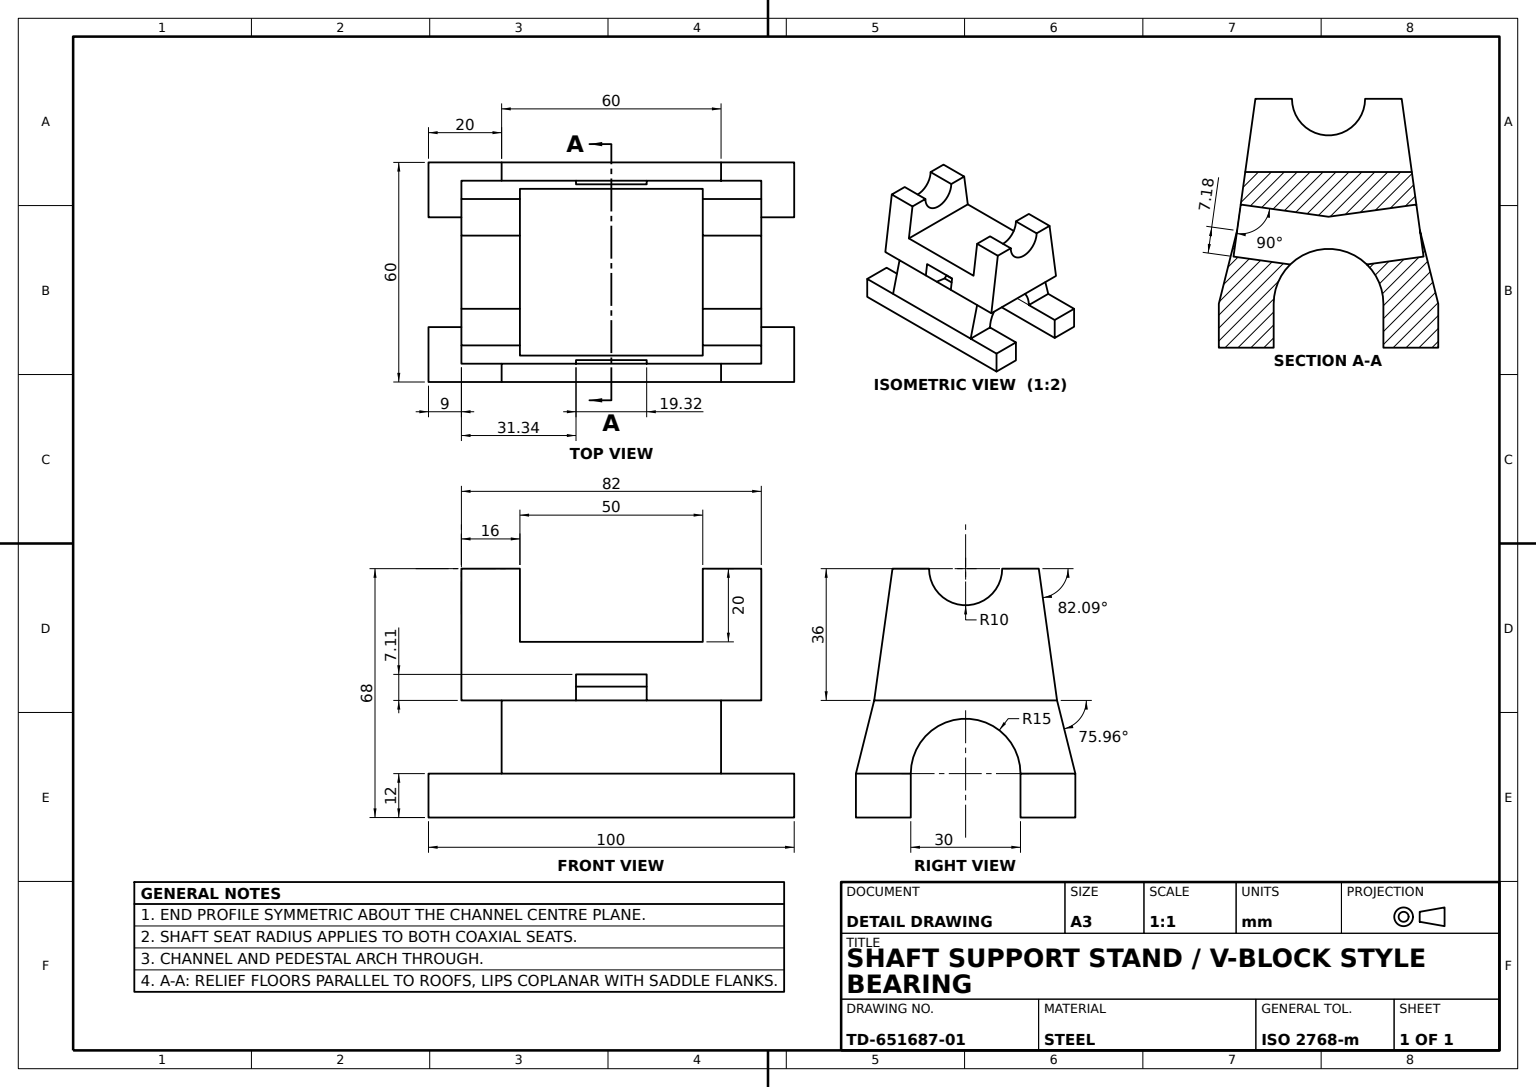
SolidWorks part; units mm, degrees
material "Plain Carbon Steel"
ref_plane "Front Plane" through (0, 0, 0) normal (0, 0, 1) x (1, 0, 0)
ref_plane "Top Plane" through (0, 0, 0) normal (0, 1, 0) x (1, 0, 0)
ref_plane "Right Plane" through (0, 0, 0) normal (1, 0, 0) x (0, 0, -1)
sketch "Base Profile Sketch" plane through (0, 0, 0) normal (0, 1, 0) x (1, 0, 0)
  line L0 (0, 0) -> (30, 0)
  line L1 (30, 0) -> (30, 100)
  line L2 (30, 100) -> (-30, 100)
  line L3 (-30, 100) -> (-30, 0)
  line L4 (-30, 0) -> (0, 0)
  dimension "D1" = 60
  dimension "D2" = 100
  dimension "D3" = 30
extrude "Base Block" add sketch "Base Profile Sketch" along normal blind 12
sketch "Base Channel Sketch" plane through (0, 12, 0) normal (0, 1, 0) x (1, 0, 0)
  line L0 (0, 0) -> (15, 0)
  line L1 (-30, 0) -> (30, 0) construction
  line L2 (15, 0) -> (15, 100)
  line L3 (30, 100) -> (-30, 100) construction
  line L4 (15, 100) -> (-15, 100)
  line L5 (-15, 100) -> (-15, 0)
  line L6 (-15, 0) -> (0, 0)
  dimension "D1" = 30
  dimension "D2" = 15
extrude "Base Channel Cut 30x15" cut sketch "Base Channel Sketch" against normal blind 73
ref_plane "Pedestal Sketch Plane" through (0, 0, -20) normal (0, 0, 1) x (1, 0, 0)
sketch "Pedestal Profile Sketch" plane through (0, 0, -20) normal (0, 0, 1) x (1, 0, 0)
  line L1 (0, 32) -> (25, 32)
  line L2 (25, 32) -> (30, 12)
  line L3 (15, 12) -> (30, 12) construction
  line L4 (0, 32) -> (-25, 32)
  line L5 (-25, 32) -> (-30, 12)
  line L6 (15, 12) -> (30, 12)
  line L7 (-30, 12) -> (-15, 12)
  arc A0 (15, 12) -> (-15, 12) centre (0, 12) ccw
  dimension "D1" = 15
  dimension "D2" = 20
  dimension "D3" = 28.072
  dimension "D4" = 32.0147
  dimension "D5" = 5
  dimension "D6" = 30
  dimension "D7" = 60
extrude "Tapered Pedestal" add sketch "Pedestal Profile Sketch" against normal blind 60
ref_plane "Saddle Sketch Plane" through (0, 0, -9) normal (0, 0, 1) x (1, 0, 0)
sketch "Saddle Profile Sketch" plane through (0, 0, -9) normal (0, 0, 1) x (1, 0, 0)
  line L0 (15, 12) -> (30, 12) construction
  line L1 (25, 32) -> (-25, 32) construction
  line L2 (10, 68) -> (20, 68)
  line L3 (20, 68) -> (25, 32)
  line L4 (25, 32) -> (-10.5729, 32)
  line L5 (-10, 68) -> (-20, 68)
  line L6 (-20, 68) -> (-25, 32)
  line L7 (-25, 32) -> (-10.5729, 32)
  arc A0 (-10, 68) -> (10, 68) centre (0, 68) ccw
  dimension "D1" = 36
  dimension "D3" = 10
  dimension "D2" = 36
  dimension "D4" = 20
  dimension "D5" = 68
  dimension "D6" = 56
  dimension "D7" = 15.814
  dimension "D8" = 10.5729
extrude "Saddle Body" add sketch "Saddle Profile Sketch" against normal blind 82
sketch "Saddle Recess Sketch" plane through (0, 68, 0) normal (0, 1, 0) x (1, 0, 0)
  line L1 (20, 91) -> (20, 9) construction
  line L2 (20, 75) -> (-20, 75)
  line L3 (-20, 91) -> (-20, 9) construction
  line L5 (-20, 25) -> (20, 25)
  line L7 (20, 75) -> (26.8933, 75)
  line L8 (26.8933, 75) -> (26.8933, 25)
  line L9 (26.8933, 25) -> (20, 25)
  line L10 (-20, 75) -> (-29.5132, 75)
  line L11 (-29.5132, 75) -> (-29.5132, 25)
  line L12 (-29.5132, 25) -> (-20, 25)
  line L13 (20, 9) -> (10, 9) construction
  dimension "D1" = 50
  dimension "D2" = 6.8933
  dimension "D3" = 49.5132
  dimension "D4" = 16
extrude "Saddle Recess Cut" cut sketch "Saddle Recess Sketch" against normal blind 20
sketch "Side Relief Sketch" plane through (28.8872, 4.0121, 0) normal (0.9905, 0.1376, 0) x (0, 0, -1)
  line L0 (80, 28.2565) -> (20, 28.2565) construction
  line L2 (40.3375, 21.0794) -> (59.6625, 21.0794)
  line L3 (40.3375, 21.0794) -> (40.3375, 35.4337)
  line L4 (40.3375, 35.4337) -> (59.6625, 35.4337)
  line L5 (59.6625, 21.0794) -> (59.6625, 35.4337)
  line L6 (40.3375, 21.0794) -> (59.6625, 35.4337) construction
  line L7 (40.3375, 35.4337) -> (59.6625, 21.0794) construction
  point P0 (50, 28.2565)
  dimension "D1" = 31.3375
  dimension "D2" = 7.1771
extrude "Side Relief Cut" cut sketch "Side Relief Sketch" against normal blind 28
mirror "Side Relief Mirror" about plane through (0, 0, 0) normal (1, 0, 0) of "Side Relief Cut"
